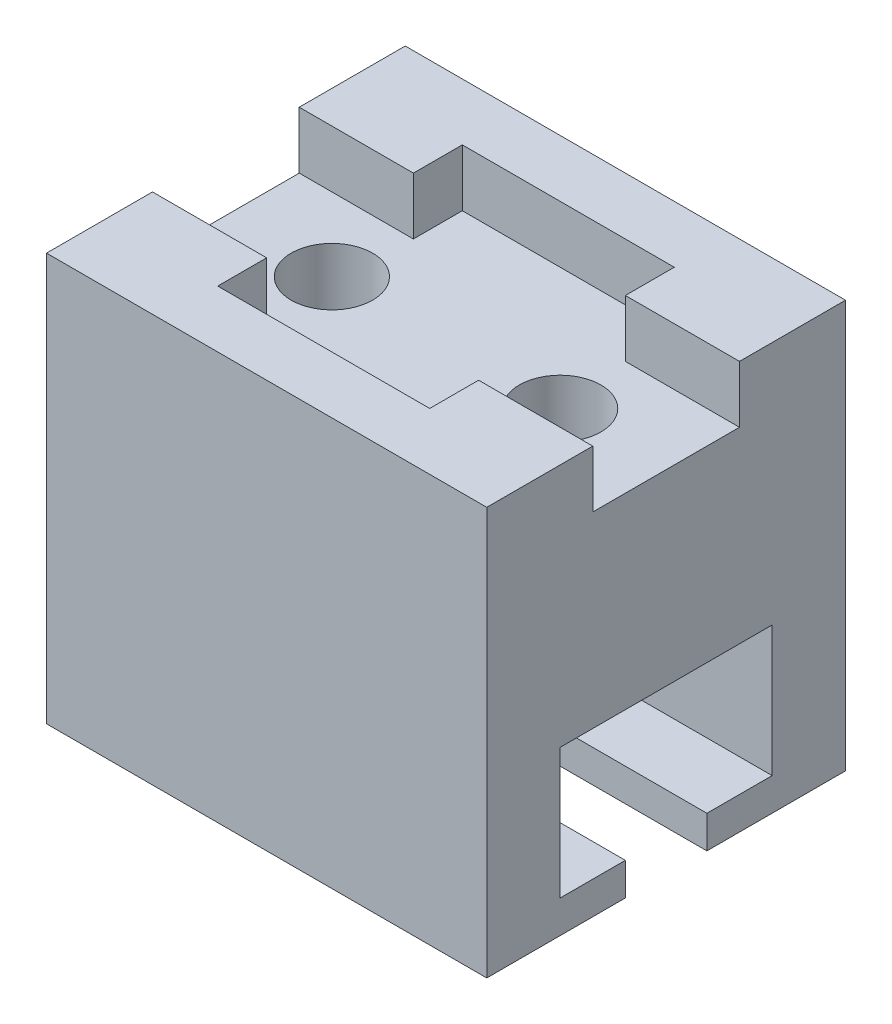
ISO-10303-21;
HEADER;
FILE_DESCRIPTION(('STEP AP214'),'2;1');
FILE_NAME('part.step','',(''),(''),'','','');
FILE_SCHEMA(('AUTOMOTIVE_DESIGN { 1 0 10303 214 1 1 1 1 }'));
ENDSEC;
DATA;
#1=APPLICATION_CONTEXT('core data for automotive mechanical design processes');
#2=APPLICATION_PROTOCOL_DEFINITION('international standard','automotive_design',2000,#1);
#3=PRODUCT_CONTEXT('',#1,'mechanical');
#4=PRODUCT('Part','Part','',(#3));
#5=PRODUCT_RELATED_PRODUCT_CATEGORY('part','',(#4));
#6=PRODUCT_DEFINITION_FORMATION('','',#4);
#7=PRODUCT_DEFINITION_CONTEXT('part definition',#1,'design');
#8=PRODUCT_DEFINITION('design','',#6,#7);
#9=PRODUCT_DEFINITION_SHAPE('','',#8);
#10=(LENGTH_UNIT() NAMED_UNIT(*) SI_UNIT(.MILLI.,.METRE.));
#11=(NAMED_UNIT(*) PLANE_ANGLE_UNIT() SI_UNIT($,.RADIAN.));
#12=(NAMED_UNIT(*) SI_UNIT($,.STERADIAN.) SOLID_ANGLE_UNIT());
#13=UNCERTAINTY_MEASURE_WITH_UNIT(LENGTH_MEASURE(1.E-05),#10,'distance_accuracy_value','');
#14=(GEOMETRIC_REPRESENTATION_CONTEXT(3) GLOBAL_UNCERTAINTY_ASSIGNED_CONTEXT((#13)) GLOBAL_UNIT_ASSIGNED_CONTEXT((#10,
#11,#12)) REPRESENTATION_CONTEXT('',''));
#15=CARTESIAN_POINT('',(0.,0.,0.));
#16=DIRECTION('',(0.,0.,1.));
#17=DIRECTION('',(1.,0.,0.));
#18=AXIS2_PLACEMENT_3D('',#15,#16,#17);
#19=CARTESIAN_POINT('',(-27.,-25.,-44.));
#20=DIRECTION('',(0.,-1.,0.));
#21=DIRECTION('',(0.,0.,-1.));
#22=AXIS2_PLACEMENT_3D('',#19,#20,#21);
#23=PLANE('',#22);
#24=DIRECTION('',(-1.,0.,0.));
#25=VECTOR('',#24,1.);
#26=CARTESIAN_POINT('',(27.,-25.,-27.));
#27=LINE('',#26,#25);
#28=CARTESIAN_POINT('',(27.,-25.,-27.));
#29=VERTEX_POINT('',#28);
#30=CARTESIAN_POINT('',(-27.,-25.,-27.));
#31=VERTEX_POINT('',#30);
#32=EDGE_CURVE('E325',#29,#31,#27,.T.);
#33=ORIENTED_EDGE('',*,*,#32,.T.);
#34=DIRECTION('',(0.,0.,1.));
#35=VECTOR('',#34,1.);
#36=CARTESIAN_POINT('',(-27.,-25.,-44.));
#37=LINE('',#36,#35);
#38=CARTESIAN_POINT('',(-27.,-25.,-44.));
#39=VERTEX_POINT('',#38);
#40=EDGE_CURVE('E223',#39,#31,#37,.T.);
#41=ORIENTED_EDGE('',*,*,#40,.F.);
#42=DIRECTION('',(1.,0.,0.));
#43=VECTOR('',#42,1.);
#44=CARTESIAN_POINT('',(-27.,-25.,-44.));
#45=LINE('',#44,#43);
#46=CARTESIAN_POINT('',(27.,-25.,-44.));
#47=VERTEX_POINT('',#46);
#48=EDGE_CURVE('E248',#39,#47,#45,.T.);
#49=ORIENTED_EDGE('',*,*,#48,.T.);
#50=DIRECTION('',(0.,0.,1.));
#51=VECTOR('',#50,1.);
#52=CARTESIAN_POINT('',(27.,-25.,-44.));
#53=LINE('',#52,#51);
#54=EDGE_CURVE('E11',#47,#29,#53,.T.);
#55=ORIENTED_EDGE('',*,*,#54,.T.);
#56=EDGE_LOOP('',(#33,#41,#49,#55));
#57=FACE_BOUND('',#56,.T.);
#58=ADVANCED_FACE('F41',(#57),#23,.T.);
#59=CARTESIAN_POINT('',(-27.,25.,-44.));
#60=DIRECTION('',(0.,1.,0.));
#61=DIRECTION('',(0.,0.,1.));
#62=AXIS2_PLACEMENT_3D('',#59,#60,#61);
#63=PLANE('',#62);
#64=DIRECTION('',(1.,0.,0.));
#65=VECTOR('',#64,1.);
#66=CARTESIAN_POINT('',(13.,25.,-13.));
#67=LINE('',#66,#65);
#68=CARTESIAN_POINT('',(13.,25.,-13.));
#69=VERTEX_POINT('',#68);
#70=CARTESIAN_POINT('',(27.,25.,-13.));
#71=VERTEX_POINT('',#70);
#72=EDGE_CURVE('E300',#69,#71,#67,.T.);
#73=ORIENTED_EDGE('',*,*,#72,.F.);
#74=DIRECTION('',(0.,0.,-1.));
#75=VECTOR('',#74,1.);
#76=CARTESIAN_POINT('',(13.,25.,-7.));
#77=LINE('',#76,#75);
#78=CARTESIAN_POINT('',(13.,25.,-7.));
#79=VERTEX_POINT('',#78);
#80=EDGE_CURVE('E303',#79,#69,#77,.T.);
#81=ORIENTED_EDGE('',*,*,#80,.F.);
#82=DIRECTION('',(1.,0.,0.));
#83=VECTOR('',#82,1.);
#84=CARTESIAN_POINT('',(-13.,25.,-7.));
#85=LINE('',#84,#83);
#86=CARTESIAN_POINT('',(-13.,25.,-7.));
#87=VERTEX_POINT('',#86);
#88=EDGE_CURVE('E305',#87,#79,#85,.T.);
#89=ORIENTED_EDGE('',*,*,#88,.F.);
#90=DIRECTION('',(0.,0.,1.));
#91=VECTOR('',#90,1.);
#92=CARTESIAN_POINT('',(-13.,25.,-7.));
#93=LINE('',#92,#91);
#94=CARTESIAN_POINT('',(-13.,25.,-13.));
#95=VERTEX_POINT('',#94);
#96=EDGE_CURVE('E307',#95,#87,#93,.T.);
#97=ORIENTED_EDGE('',*,*,#96,.F.);
#98=DIRECTION('',(1.,0.,0.));
#99=VECTOR('',#98,1.);
#100=CARTESIAN_POINT('',(-27.,25.,-13.));
#101=LINE('',#100,#99);
#102=CARTESIAN_POINT('',(-27.,25.,-13.));
#103=VERTEX_POINT('',#102);
#104=EDGE_CURVE('E309',#103,#95,#101,.T.);
#105=ORIENTED_EDGE('',*,*,#104,.F.);
#106=DIRECTION('',(0.,0.,1.));
#107=VECTOR('',#106,1.);
#108=CARTESIAN_POINT('',(-27.,25.,-44.));
#109=LINE('',#108,#107);
#110=CARTESIAN_POINT('',(-27.,25.,0.));
#111=VERTEX_POINT('',#110);
#112=EDGE_CURVE('E232',#103,#111,#109,.T.);
#113=ORIENTED_EDGE('',*,*,#112,.T.);
#114=DIRECTION('',(-1.,0.,0.));
#115=VECTOR('',#114,1.);
#116=CARTESIAN_POINT('',(-27.,25.,0.));
#117=LINE('',#116,#115);
#118=CARTESIAN_POINT('',(27.,25.,0.));
#119=VERTEX_POINT('',#118);
#120=EDGE_CURVE('E257',#119,#111,#117,.T.);
#121=ORIENTED_EDGE('',*,*,#120,.F.);
#122=DIRECTION('',(0.,0.,1.));
#123=VECTOR('',#122,1.);
#124=CARTESIAN_POINT('',(27.,25.,-44.));
#125=LINE('',#124,#123);
#126=EDGE_CURVE('E242',#71,#119,#125,.T.);
#127=ORIENTED_EDGE('',*,*,#126,.F.);
#128=EDGE_LOOP('',(#73,#81,#89,#97,#105,#113,#121,#127));
#129=FACE_BOUND('',#128,.T.);
#130=ADVANCED_FACE('F448',(#129),#63,.T.);
#131=CARTESIAN_POINT('',(27.,-25.,-44.));
#132=DIRECTION('',(1.,0.,0.));
#133=DIRECTION('',(0.,0.,-1.));
#134=AXIS2_PLACEMENT_3D('',#131,#132,#133);
#135=PLANE('',#134);
#136=DIRECTION('',(0.,-1.,0.));
#137=VECTOR('',#136,1.);
#138=CARTESIAN_POINT('',(27.,-25.,-27.));
#139=LINE('',#138,#137);
#140=CARTESIAN_POINT('',(27.,-21.,-27.));
#141=VERTEX_POINT('',#140);
#142=EDGE_CURVE('E218',#141,#29,#139,.T.);
#143=ORIENTED_EDGE('',*,*,#142,.T.);
#144=ORIENTED_EDGE('',*,*,#54,.F.);
#145=DIRECTION('',(0.,1.,0.));
#146=VECTOR('',#145,1.);
#147=CARTESIAN_POINT('',(27.,-25.,-44.));
#148=LINE('',#147,#146);
#149=CARTESIAN_POINT('',(27.,25.,-44.));
#150=VERTEX_POINT('',#149);
#151=EDGE_CURVE('E266',#47,#150,#148,.T.);
#152=ORIENTED_EDGE('',*,*,#151,.T.);
#153=CARTESIAN_POINT('',(27.,25.,-31.));
#154=VERTEX_POINT('',#153);
#155=EDGE_CURVE('E44',#150,#154,#125,.T.);
#156=ORIENTED_EDGE('',*,*,#155,.T.);
#157=DIRECTION('',(0.,1.,0.));
#158=VECTOR('',#157,1.);
#159=CARTESIAN_POINT('',(27.,18.,-31.));
#160=LINE('',#159,#158);
#161=CARTESIAN_POINT('',(27.,18.,-31.));
#162=VERTEX_POINT('',#161);
#163=EDGE_CURVE('E295',#162,#154,#160,.T.);
#164=ORIENTED_EDGE('',*,*,#163,.F.);
#165=DIRECTION('',(0.,0.,-1.));
#166=VECTOR('',#165,1.);
#167=CARTESIAN_POINT('',(27.,18.,-31.));
#168=LINE('',#167,#166);
#169=CARTESIAN_POINT('',(27.,18.,-13.));
#170=VERTEX_POINT('',#169);
#171=EDGE_CURVE('E324',#170,#162,#168,.T.);
#172=ORIENTED_EDGE('',*,*,#171,.F.);
#173=DIRECTION('',(0.,1.,0.));
#174=VECTOR('',#173,1.);
#175=CARTESIAN_POINT('',(27.,18.,-13.));
#176=LINE('',#175,#174);
#177=EDGE_CURVE('E286',#170,#71,#176,.T.);
#178=ORIENTED_EDGE('',*,*,#177,.T.);
#179=ORIENTED_EDGE('',*,*,#126,.T.);
#180=DIRECTION('',(0.,1.,0.));
#181=VECTOR('',#180,1.);
#182=CARTESIAN_POINT('',(27.,-25.,0.));
#183=LINE('',#182,#181);
#184=CARTESIAN_POINT('',(27.,-25.,0.));
#185=VERTEX_POINT('',#184);
#186=EDGE_CURVE('E224',#185,#119,#183,.T.);
#187=ORIENTED_EDGE('',*,*,#186,.F.);
#188=CARTESIAN_POINT('',(27.,-25.,-17.));
#189=VERTEX_POINT('',#188);
#190=EDGE_CURVE('E49',#189,#185,#53,.T.);
#191=ORIENTED_EDGE('',*,*,#190,.F.);
#192=DIRECTION('',(0.,1.,0.));
#193=VECTOR('',#192,1.);
#194=CARTESIAN_POINT('',(27.,-21.,-17.));
#195=LINE('',#194,#193);
#196=CARTESIAN_POINT('',(27.,-21.,-17.));
#197=VERTEX_POINT('',#196);
#198=EDGE_CURVE('E201',#189,#197,#195,.T.);
#199=ORIENTED_EDGE('',*,*,#198,.T.);
#200=DIRECTION('',(0.,0.,1.));
#201=VECTOR('',#200,1.);
#202=CARTESIAN_POINT('',(27.,-21.,-9.));
#203=LINE('',#202,#201);
#204=CARTESIAN_POINT('',(27.,-21.,-9.));
#205=VERTEX_POINT('',#204);
#206=EDGE_CURVE('E209',#197,#205,#203,.T.);
#207=ORIENTED_EDGE('',*,*,#206,.T.);
#208=DIRECTION('',(0.,1.,0.));
#209=VECTOR('',#208,1.);
#210=CARTESIAN_POINT('',(27.,-5.,-9.));
#211=LINE('',#210,#209);
#212=CARTESIAN_POINT('',(27.,-5.,-9.));
#213=VERTEX_POINT('',#212);
#214=EDGE_CURVE('E397',#205,#213,#211,.T.);
#215=ORIENTED_EDGE('',*,*,#214,.T.);
#216=DIRECTION('',(0.,0.,-1.));
#217=VECTOR('',#216,1.);
#218=CARTESIAN_POINT('',(27.,-5.,-35.));
#219=LINE('',#218,#217);
#220=CARTESIAN_POINT('',(27.,-5.,-35.));
#221=VERTEX_POINT('',#220);
#222=EDGE_CURVE('E391',#213,#221,#219,.T.);
#223=ORIENTED_EDGE('',*,*,#222,.T.);
#224=DIRECTION('',(0.,-1.,0.));
#225=VECTOR('',#224,1.);
#226=CARTESIAN_POINT('',(27.,-21.,-35.));
#227=LINE('',#226,#225);
#228=CARTESIAN_POINT('',(27.,-21.,-35.));
#229=VERTEX_POINT('',#228);
#230=EDGE_CURVE('E394',#221,#229,#227,.T.);
#231=ORIENTED_EDGE('',*,*,#230,.T.);
#232=DIRECTION('',(0.,0.,1.));
#233=VECTOR('',#232,1.);
#234=CARTESIAN_POINT('',(27.,-21.,-27.));
#235=LINE('',#234,#233);
#236=EDGE_CURVE('E386',#229,#141,#235,.T.);
#237=ORIENTED_EDGE('',*,*,#236,.T.);
#238=EDGE_LOOP('',(#143,#144,#152,#156,#164,#172,#178,#179,#187,#191,#199,#207,#215,#223,#231,#237));
#239=FACE_BOUND('',#238,.T.);
#240=ADVANCED_FACE('F43',(#239),#135,.T.);
#241=DIRECTION('',(-1.,0.,0.));
#242=VECTOR('',#241,1.);
#243=CARTESIAN_POINT('',(27.,-25.,-17.));
#244=LINE('',#243,#242);
#245=CARTESIAN_POINT('',(-27.,-25.,-17.));
#246=VERTEX_POINT('',#245);
#247=EDGE_CURVE('E59',#189,#246,#244,.T.);
#248=ORIENTED_EDGE('',*,*,#247,.F.);
#249=ORIENTED_EDGE('',*,*,#190,.T.);
#250=DIRECTION('',(1.,0.,0.));
#251=VECTOR('',#250,1.);
#252=CARTESIAN_POINT('',(-27.,-25.,0.));
#253=LINE('',#252,#251);
#254=CARTESIAN_POINT('',(-27.,-25.,0.));
#255=VERTEX_POINT('',#254);
#256=EDGE_CURVE('E230',#255,#185,#253,.T.);
#257=ORIENTED_EDGE('',*,*,#256,.F.);
#258=EDGE_CURVE('E217',#246,#255,#37,.T.);
#259=ORIENTED_EDGE('',*,*,#258,.F.);
#260=EDGE_LOOP('',(#248,#249,#257,#259));
#261=FACE_BOUND('',#260,.T.);
#262=ADVANCED_FACE('F214',(#261),#23,.T.);
#263=CARTESIAN_POINT('',(-27.,-25.,-44.));
#264=DIRECTION('',(-1.,0.,0.));
#265=DIRECTION('',(0.,0.,1.));
#266=AXIS2_PLACEMENT_3D('',#263,#264,#265);
#267=PLANE('',#266);
#268=DIRECTION('',(0.,-1.,0.));
#269=VECTOR('',#268,1.);
#270=CARTESIAN_POINT('',(-27.,-25.,-27.));
#271=LINE('',#270,#269);
#272=CARTESIAN_POINT('',(-27.,-21.,-27.));
#273=VERTEX_POINT('',#272);
#274=EDGE_CURVE('E211',#273,#31,#271,.T.);
#275=ORIENTED_EDGE('',*,*,#274,.F.);
#276=DIRECTION('',(0.,0.,1.));
#277=VECTOR('',#276,1.);
#278=CARTESIAN_POINT('',(-27.,-21.,-27.));
#279=LINE('',#278,#277);
#280=CARTESIAN_POINT('',(-27.,-21.,-35.));
#281=VERTEX_POINT('',#280);
#282=EDGE_CURVE('E367',#281,#273,#279,.T.);
#283=ORIENTED_EDGE('',*,*,#282,.F.);
#284=DIRECTION('',(0.,-1.,0.));
#285=VECTOR('',#284,1.);
#286=CARTESIAN_POINT('',(-27.,-21.,-35.));
#287=LINE('',#286,#285);
#288=CARTESIAN_POINT('',(-27.,-5.,-35.));
#289=VERTEX_POINT('',#288);
#290=EDGE_CURVE('E373',#289,#281,#287,.T.);
#291=ORIENTED_EDGE('',*,*,#290,.F.);
#292=DIRECTION('',(0.,0.,-1.));
#293=VECTOR('',#292,1.);
#294=CARTESIAN_POINT('',(-27.,-5.,-35.));
#295=LINE('',#294,#293);
#296=CARTESIAN_POINT('',(-27.,-5.,-9.));
#297=VERTEX_POINT('',#296);
#298=EDGE_CURVE('E376',#297,#289,#295,.T.);
#299=ORIENTED_EDGE('',*,*,#298,.F.);
#300=DIRECTION('',(0.,1.,0.));
#301=VECTOR('',#300,1.);
#302=CARTESIAN_POINT('',(-27.,-5.,-9.));
#303=LINE('',#302,#301);
#304=CARTESIAN_POINT('',(-27.,-21.,-9.));
#305=VERTEX_POINT('',#304);
#306=EDGE_CURVE('E377',#305,#297,#303,.T.);
#307=ORIENTED_EDGE('',*,*,#306,.F.);
#308=DIRECTION('',(0.,0.,1.));
#309=VECTOR('',#308,1.);
#310=CARTESIAN_POINT('',(-27.,-21.,-9.));
#311=LINE('',#310,#309);
#312=CARTESIAN_POINT('',(-27.,-21.,-17.));
#313=VERTEX_POINT('',#312);
#314=EDGE_CURVE('E385',#313,#305,#311,.T.);
#315=ORIENTED_EDGE('',*,*,#314,.F.);
#316=DIRECTION('',(0.,1.,0.));
#317=VECTOR('',#316,1.);
#318=CARTESIAN_POINT('',(-27.,-21.,-17.));
#319=LINE('',#318,#317);
#320=EDGE_CURVE('E384',#246,#313,#319,.T.);
#321=ORIENTED_EDGE('',*,*,#320,.F.);
#322=ORIENTED_EDGE('',*,*,#258,.T.);
#323=DIRECTION('',(0.,-1.,0.));
#324=VECTOR('',#323,1.);
#325=CARTESIAN_POINT('',(-27.,-25.,0.));
#326=LINE('',#325,#324);
#327=EDGE_CURVE('E263',#111,#255,#326,.T.);
#328=ORIENTED_EDGE('',*,*,#327,.F.);
#329=ORIENTED_EDGE('',*,*,#112,.F.);
#330=DIRECTION('',(0.,1.,0.));
#331=VECTOR('',#330,1.);
#332=CARTESIAN_POINT('',(-27.,18.,-13.));
#333=LINE('',#332,#331);
#334=CARTESIAN_POINT('',(-27.,18.,-13.));
#335=VERTEX_POINT('',#334);
#336=EDGE_CURVE('E278',#335,#103,#333,.T.);
#337=ORIENTED_EDGE('',*,*,#336,.F.);
#338=DIRECTION('',(0.,0.,1.));
#339=VECTOR('',#338,1.);
#340=CARTESIAN_POINT('',(-27.,18.,-31.));
#341=LINE('',#340,#339);
#342=CARTESIAN_POINT('',(-27.,18.,-31.));
#343=VERTEX_POINT('',#342);
#344=EDGE_CURVE('E344',#343,#335,#341,.T.);
#345=ORIENTED_EDGE('',*,*,#344,.F.);
#346=DIRECTION('',(0.,1.,0.));
#347=VECTOR('',#346,1.);
#348=CARTESIAN_POINT('',(-27.,18.,-31.));
#349=LINE('',#348,#347);
#350=CARTESIAN_POINT('',(-27.,25.,-31.));
#351=VERTEX_POINT('',#350);
#352=EDGE_CURVE('E280',#343,#351,#349,.T.);
#353=ORIENTED_EDGE('',*,*,#352,.T.);
#354=CARTESIAN_POINT('',(-27.,25.,-44.));
#355=VERTEX_POINT('',#354);
#356=EDGE_CURVE('E233',#355,#351,#109,.T.);
#357=ORIENTED_EDGE('',*,*,#356,.F.);
#358=DIRECTION('',(0.,-1.,0.));
#359=VECTOR('',#358,1.);
#360=CARTESIAN_POINT('',(-27.,-25.,-44.));
#361=LINE('',#360,#359);
#362=EDGE_CURVE('E246',#355,#39,#361,.T.);
#363=ORIENTED_EDGE('',*,*,#362,.T.);
#364=ORIENTED_EDGE('',*,*,#40,.T.);
#365=EDGE_LOOP('',(#275,#283,#291,#299,#307,#315,#321,#322,#328,#329,#337,#345,#353,#357,#363,#364));
#366=FACE_BOUND('',#365,.T.);
#367=ADVANCED_FACE('F442',(#366),#267,.T.);
#368=DIRECTION('',(-1.,0.,0.));
#369=VECTOR('',#368,1.);
#370=CARTESIAN_POINT('',(13.,25.,-31.));
#371=LINE('',#370,#369);
#372=CARTESIAN_POINT('',(13.,25.,-31.));
#373=VERTEX_POINT('',#372);
#374=EDGE_CURVE('E293',#154,#373,#371,.T.);
#375=ORIENTED_EDGE('',*,*,#374,.F.);
#376=ORIENTED_EDGE('',*,*,#155,.F.);
#377=DIRECTION('',(-1.,0.,0.));
#378=VECTOR('',#377,1.);
#379=CARTESIAN_POINT('',(-27.,25.,-44.));
#380=LINE('',#379,#378);
#381=EDGE_CURVE('E254',#150,#355,#380,.T.);
#382=ORIENTED_EDGE('',*,*,#381,.T.);
#383=ORIENTED_EDGE('',*,*,#356,.T.);
#384=DIRECTION('',(-1.,0.,0.));
#385=VECTOR('',#384,1.);
#386=CARTESIAN_POINT('',(-27.,25.,-31.));
#387=LINE('',#386,#385);
#388=CARTESIAN_POINT('',(-13.,25.,-31.));
#389=VERTEX_POINT('',#388);
#390=EDGE_CURVE('E311',#389,#351,#387,.T.);
#391=ORIENTED_EDGE('',*,*,#390,.F.);
#392=DIRECTION('',(0.,0.,1.));
#393=VECTOR('',#392,1.);
#394=CARTESIAN_POINT('',(-13.,25.,-37.));
#395=LINE('',#394,#393);
#396=CARTESIAN_POINT('',(-13.,25.,-37.));
#397=VERTEX_POINT('',#396);
#398=EDGE_CURVE('E312',#397,#389,#395,.T.);
#399=ORIENTED_EDGE('',*,*,#398,.F.);
#400=DIRECTION('',(-1.,0.,0.));
#401=VECTOR('',#400,1.);
#402=CARTESIAN_POINT('',(-13.,25.,-37.));
#403=LINE('',#402,#401);
#404=CARTESIAN_POINT('',(13.,25.,-37.));
#405=VERTEX_POINT('',#404);
#406=EDGE_CURVE('E318',#405,#397,#403,.T.);
#407=ORIENTED_EDGE('',*,*,#406,.F.);
#408=DIRECTION('',(0.,0.,-1.));
#409=VECTOR('',#408,1.);
#410=CARTESIAN_POINT('',(13.,25.,-37.));
#411=LINE('',#410,#409);
#412=EDGE_CURVE('E68',#373,#405,#411,.T.);
#413=ORIENTED_EDGE('',*,*,#412,.F.);
#414=EDGE_LOOP('',(#375,#376,#382,#383,#391,#399,#407,#413));
#415=FACE_BOUND('',#414,.T.);
#416=ADVANCED_FACE('F461',(#415),#63,.T.);
#417=CARTESIAN_POINT('',(0.,0.,-44.));
#418=DIRECTION('',(0.,0.,-1.));
#419=DIRECTION('',(-1.,0.,0.));
#420=AXIS2_PLACEMENT_3D('',#417,#418,#419);
#421=PLANE('',#420);
#422=ORIENTED_EDGE('',*,*,#151,.F.);
#423=ORIENTED_EDGE('',*,*,#48,.F.);
#424=ORIENTED_EDGE('',*,*,#362,.F.);
#425=ORIENTED_EDGE('',*,*,#381,.F.);
#426=EDGE_LOOP('',(#422,#423,#424,#425));
#427=FACE_BOUND('',#426,.T.);
#428=ADVANCED_FACE('F640',(#427),#421,.T.);
#429=CARTESIAN_POINT('',(0.,0.,0.));
#430=DIRECTION('',(0.,0.,-1.));
#431=DIRECTION('',(-1.,0.,0.));
#432=AXIS2_PLACEMENT_3D('',#429,#430,#431);
#433=PLANE('',#432);
#434=ORIENTED_EDGE('',*,*,#186,.T.);
#435=ORIENTED_EDGE('',*,*,#120,.T.);
#436=ORIENTED_EDGE('',*,*,#327,.T.);
#437=ORIENTED_EDGE('',*,*,#256,.T.);
#438=EDGE_LOOP('',(#434,#435,#436,#437));
#439=FACE_BOUND('',#438,.T.);
#440=ADVANCED_FACE('F636',(#439),#433,.F.);
#441=CARTESIAN_POINT('',(13.,18.,-37.));
#442=DIRECTION('',(1.,0.,0.));
#443=DIRECTION('',(0.,0.,-1.));
#444=AXIS2_PLACEMENT_3D('',#441,#442,#443);
#445=PLANE('',#444);
#446=ORIENTED_EDGE('',*,*,#412,.T.);
#447=DIRECTION('',(0.,1.,0.));
#448=VECTOR('',#447,1.);
#449=CARTESIAN_POINT('',(13.,18.,-37.));
#450=LINE('',#449,#448);
#451=CARTESIAN_POINT('',(13.,18.,-37.));
#452=VERTEX_POINT('',#451);
#453=EDGE_CURVE('E269',#452,#405,#450,.T.);
#454=ORIENTED_EDGE('',*,*,#453,.F.);
#455=DIRECTION('',(0.,0.,-1.));
#456=VECTOR('',#455,1.);
#457=CARTESIAN_POINT('',(13.,18.,-37.));
#458=LINE('',#457,#456);
#459=CARTESIAN_POINT('',(13.,18.,-31.));
#460=VERTEX_POINT('',#459);
#461=EDGE_CURVE('E297',#460,#452,#458,.T.);
#462=ORIENTED_EDGE('',*,*,#461,.F.);
#463=DIRECTION('',(0.,1.,0.));
#464=VECTOR('',#463,1.);
#465=CARTESIAN_POINT('',(13.,18.,-31.));
#466=LINE('',#465,#464);
#467=EDGE_CURVE('E261',#460,#373,#466,.T.);
#468=ORIENTED_EDGE('',*,*,#467,.T.);
#469=EDGE_LOOP('',(#446,#454,#462,#468));
#470=FACE_BOUND('',#469,.T.);
#471=ADVANCED_FACE('F428',(#470),#445,.F.);
#472=CARTESIAN_POINT('',(13.,18.,-31.));
#473=DIRECTION('',(0.,0.,-1.));
#474=DIRECTION('',(-1.,0.,0.));
#475=AXIS2_PLACEMENT_3D('',#472,#473,#474);
#476=PLANE('',#475);
#477=ORIENTED_EDGE('',*,*,#374,.T.);
#478=ORIENTED_EDGE('',*,*,#467,.F.);
#479=DIRECTION('',(-1.,0.,0.));
#480=VECTOR('',#479,1.);
#481=CARTESIAN_POINT('',(13.,18.,-31.));
#482=LINE('',#481,#480);
#483=EDGE_CURVE('E272',#162,#460,#482,.T.);
#484=ORIENTED_EDGE('',*,*,#483,.F.);
#485=ORIENTED_EDGE('',*,*,#163,.T.);
#486=EDGE_LOOP('',(#477,#478,#484,#485));
#487=FACE_BOUND('',#486,.T.);
#488=ADVANCED_FACE('F465',(#487),#476,.F.);
#489=CARTESIAN_POINT('',(13.,18.,-13.));
#490=DIRECTION('',(0.,0.,1.));
#491=DIRECTION('',(1.,0.,0.));
#492=AXIS2_PLACEMENT_3D('',#489,#490,#491);
#493=PLANE('',#492);
#494=ORIENTED_EDGE('',*,*,#72,.T.);
#495=ORIENTED_EDGE('',*,*,#177,.F.);
#496=DIRECTION('',(1.,0.,0.));
#497=VECTOR('',#496,1.);
#498=CARTESIAN_POINT('',(13.,18.,-13.));
#499=LINE('',#498,#497);
#500=CARTESIAN_POINT('',(13.,18.,-13.));
#501=VERTEX_POINT('',#500);
#502=EDGE_CURVE('E330',#501,#170,#499,.T.);
#503=ORIENTED_EDGE('',*,*,#502,.F.);
#504=DIRECTION('',(0.,1.,0.));
#505=VECTOR('',#504,1.);
#506=CARTESIAN_POINT('',(13.,18.,-13.));
#507=LINE('',#506,#505);
#508=EDGE_CURVE('E287',#501,#69,#507,.T.);
#509=ORIENTED_EDGE('',*,*,#508,.T.);
#510=EDGE_LOOP('',(#494,#495,#503,#509));
#511=FACE_BOUND('',#510,.T.);
#512=ADVANCED_FACE('F458',(#511),#493,.F.);
#513=CARTESIAN_POINT('',(13.,18.,-7.));
#514=DIRECTION('',(1.,0.,0.));
#515=DIRECTION('',(0.,0.,-1.));
#516=AXIS2_PLACEMENT_3D('',#513,#514,#515);
#517=PLANE('',#516);
#518=ORIENTED_EDGE('',*,*,#80,.T.);
#519=ORIENTED_EDGE('',*,*,#508,.F.);
#520=DIRECTION('',(0.,0.,-1.));
#521=VECTOR('',#520,1.);
#522=CARTESIAN_POINT('',(13.,18.,-7.));
#523=LINE('',#522,#521);
#524=CARTESIAN_POINT('',(13.,18.,-7.));
#525=VERTEX_POINT('',#524);
#526=EDGE_CURVE('E329',#525,#501,#523,.T.);
#527=ORIENTED_EDGE('',*,*,#526,.F.);
#528=DIRECTION('',(0.,1.,0.));
#529=VECTOR('',#528,1.);
#530=CARTESIAN_POINT('',(13.,18.,-7.));
#531=LINE('',#530,#529);
#532=EDGE_CURVE('E288',#525,#79,#531,.T.);
#533=ORIENTED_EDGE('',*,*,#532,.T.);
#534=EDGE_LOOP('',(#518,#519,#527,#533));
#535=FACE_BOUND('',#534,.T.);
#536=ADVANCED_FACE('F460',(#535),#517,.F.);
#537=CARTESIAN_POINT('',(-13.,18.,-7.));
#538=DIRECTION('',(0.,0.,1.));
#539=DIRECTION('',(1.,0.,0.));
#540=AXIS2_PLACEMENT_3D('',#537,#538,#539);
#541=PLANE('',#540);
#542=ORIENTED_EDGE('',*,*,#88,.T.);
#543=ORIENTED_EDGE('',*,*,#532,.F.);
#544=DIRECTION('',(1.,0.,0.));
#545=VECTOR('',#544,1.);
#546=CARTESIAN_POINT('',(-13.,18.,-7.));
#547=LINE('',#546,#545);
#548=CARTESIAN_POINT('',(-13.,18.,-7.));
#549=VERTEX_POINT('',#548);
#550=EDGE_CURVE('E334',#549,#525,#547,.T.);
#551=ORIENTED_EDGE('',*,*,#550,.F.);
#552=DIRECTION('',(0.,1.,0.));
#553=VECTOR('',#552,1.);
#554=CARTESIAN_POINT('',(-13.,18.,-7.));
#555=LINE('',#554,#553);
#556=EDGE_CURVE('E285',#549,#87,#555,.T.);
#557=ORIENTED_EDGE('',*,*,#556,.T.);
#558=EDGE_LOOP('',(#542,#543,#551,#557));
#559=FACE_BOUND('',#558,.T.);
#560=ADVANCED_FACE('F451',(#559),#541,.F.);
#561=CARTESIAN_POINT('',(-13.,18.,-7.));
#562=DIRECTION('',(-1.,0.,0.));
#563=DIRECTION('',(0.,0.,1.));
#564=AXIS2_PLACEMENT_3D('',#561,#562,#563);
#565=PLANE('',#564);
#566=ORIENTED_EDGE('',*,*,#96,.T.);
#567=ORIENTED_EDGE('',*,*,#556,.F.);
#568=DIRECTION('',(0.,0.,1.));
#569=VECTOR('',#568,1.);
#570=CARTESIAN_POINT('',(-13.,18.,-7.));
#571=LINE('',#570,#569);
#572=CARTESIAN_POINT('',(-13.,18.,-13.));
#573=VERTEX_POINT('',#572);
#574=EDGE_CURVE('E338',#573,#549,#571,.T.);
#575=ORIENTED_EDGE('',*,*,#574,.F.);
#576=DIRECTION('',(0.,1.,0.));
#577=VECTOR('',#576,1.);
#578=CARTESIAN_POINT('',(-13.,18.,-13.));
#579=LINE('',#578,#577);
#580=EDGE_CURVE('E284',#573,#95,#579,.T.);
#581=ORIENTED_EDGE('',*,*,#580,.T.);
#582=EDGE_LOOP('',(#566,#567,#575,#581));
#583=FACE_BOUND('',#582,.T.);
#584=ADVANCED_FACE('F446',(#583),#565,.F.);
#585=CARTESIAN_POINT('',(-27.,18.,-13.));
#586=DIRECTION('',(0.,0.,1.));
#587=DIRECTION('',(1.,0.,0.));
#588=AXIS2_PLACEMENT_3D('',#585,#586,#587);
#589=PLANE('',#588);
#590=ORIENTED_EDGE('',*,*,#104,.T.);
#591=ORIENTED_EDGE('',*,*,#580,.F.);
#592=DIRECTION('',(1.,0.,0.));
#593=VECTOR('',#592,1.);
#594=CARTESIAN_POINT('',(-27.,18.,-13.));
#595=LINE('',#594,#593);
#596=EDGE_CURVE('E340',#335,#573,#595,.T.);
#597=ORIENTED_EDGE('',*,*,#596,.F.);
#598=ORIENTED_EDGE('',*,*,#336,.T.);
#599=EDGE_LOOP('',(#590,#591,#597,#598));
#600=FACE_BOUND('',#599,.T.);
#601=ADVANCED_FACE('F444',(#600),#589,.F.);
#602=CARTESIAN_POINT('',(-27.,18.,-31.));
#603=DIRECTION('',(0.,0.,-1.));
#604=DIRECTION('',(-1.,0.,0.));
#605=AXIS2_PLACEMENT_3D('',#602,#603,#604);
#606=PLANE('',#605);
#607=ORIENTED_EDGE('',*,*,#390,.T.);
#608=ORIENTED_EDGE('',*,*,#352,.F.);
#609=DIRECTION('',(-1.,0.,0.));
#610=VECTOR('',#609,1.);
#611=CARTESIAN_POINT('',(-27.,18.,-31.));
#612=LINE('',#611,#610);
#613=CARTESIAN_POINT('',(-13.,18.,-31.));
#614=VERTEX_POINT('',#613);
#615=EDGE_CURVE('E341',#614,#343,#612,.T.);
#616=ORIENTED_EDGE('',*,*,#615,.F.);
#617=DIRECTION('',(0.,1.,0.));
#618=VECTOR('',#617,1.);
#619=CARTESIAN_POINT('',(-13.,18.,-31.));
#620=LINE('',#619,#618);
#621=EDGE_CURVE('E274',#614,#389,#620,.T.);
#622=ORIENTED_EDGE('',*,*,#621,.T.);
#623=EDGE_LOOP('',(#607,#608,#616,#622));
#624=FACE_BOUND('',#623,.T.);
#625=ADVANCED_FACE('F469',(#624),#606,.F.);
#626=CARTESIAN_POINT('',(-13.,18.,-37.));
#627=DIRECTION('',(-1.,0.,0.));
#628=DIRECTION('',(0.,0.,1.));
#629=AXIS2_PLACEMENT_3D('',#626,#627,#628);
#630=PLANE('',#629);
#631=ORIENTED_EDGE('',*,*,#398,.T.);
#632=ORIENTED_EDGE('',*,*,#621,.F.);
#633=DIRECTION('',(0.,0.,1.));
#634=VECTOR('',#633,1.);
#635=CARTESIAN_POINT('',(-13.,18.,-37.));
#636=LINE('',#635,#634);
#637=CARTESIAN_POINT('',(-13.,18.,-37.));
#638=VERTEX_POINT('',#637);
#639=EDGE_CURVE('E346',#638,#614,#636,.T.);
#640=ORIENTED_EDGE('',*,*,#639,.F.);
#641=DIRECTION('',(0.,1.,0.));
#642=VECTOR('',#641,1.);
#643=CARTESIAN_POINT('',(-13.,18.,-37.));
#644=LINE('',#643,#642);
#645=EDGE_CURVE('E275',#638,#397,#644,.T.);
#646=ORIENTED_EDGE('',*,*,#645,.T.);
#647=EDGE_LOOP('',(#631,#632,#640,#646));
#648=FACE_BOUND('',#647,.T.);
#649=ADVANCED_FACE('F432',(#648),#630,.F.);
#650=CARTESIAN_POINT('',(-13.,18.,-37.));
#651=DIRECTION('',(0.,0.,-1.));
#652=DIRECTION('',(-1.,0.,0.));
#653=AXIS2_PLACEMENT_3D('',#650,#651,#652);
#654=PLANE('',#653);
#655=ORIENTED_EDGE('',*,*,#406,.T.);
#656=ORIENTED_EDGE('',*,*,#645,.F.);
#657=DIRECTION('',(-1.,0.,0.));
#658=VECTOR('',#657,1.);
#659=CARTESIAN_POINT('',(-13.,18.,-37.));
#660=LINE('',#659,#658);
#661=EDGE_CURVE('E353',#452,#638,#660,.T.);
#662=ORIENTED_EDGE('',*,*,#661,.F.);
#663=ORIENTED_EDGE('',*,*,#453,.T.);
#664=EDGE_LOOP('',(#655,#656,#662,#663));
#665=FACE_BOUND('',#664,.T.);
#666=ADVANCED_FACE('F423',(#665),#654,.F.);
#667=CARTESIAN_POINT('',(0.,18.,0.));
#668=DIRECTION('',(0.,1.,0.));
#669=DIRECTION('',(0.,0.,1.));
#670=AXIS2_PLACEMENT_3D('',#667,#668,#669);
#671=PLANE('',#670);
#672=CARTESIAN_POINT('',(-14.,18.,-22.));
#673=DIRECTION('',(0.,1.,0.));
#674=DIRECTION('',(0.,0.,1.));
#675=AXIS2_PLACEMENT_3D('',#672,#673,#674);
#676=CIRCLE('',#675,5.);
#677=CARTESIAN_POINT('',(-14.,18.,-17.));
#678=VERTEX_POINT('',#677);
#679=EDGE_CURVE('E409',#678,#678,#676,.T.);
#680=ORIENTED_EDGE('',*,*,#679,.F.);
#681=EDGE_LOOP('',(#680));
#682=FACE_BOUND('',#681,.T.);
#683=CARTESIAN_POINT('',(14.,18.,-22.));
#684=DIRECTION('',(0.,1.,0.));
#685=DIRECTION('',(0.,0.,1.));
#686=AXIS2_PLACEMENT_3D('',#683,#684,#685);
#687=CIRCLE('',#686,5.);
#688=CARTESIAN_POINT('',(14.,18.,-17.));
#689=VERTEX_POINT('',#688);
#690=EDGE_CURVE('E407',#689,#689,#687,.T.);
#691=ORIENTED_EDGE('',*,*,#690,.F.);
#692=EDGE_LOOP('',(#691));
#693=FACE_BOUND('',#692,.T.);
#694=ORIENTED_EDGE('',*,*,#461,.T.);
#695=ORIENTED_EDGE('',*,*,#661,.T.);
#696=ORIENTED_EDGE('',*,*,#639,.T.);
#697=ORIENTED_EDGE('',*,*,#615,.T.);
#698=ORIENTED_EDGE('',*,*,#344,.T.);
#699=ORIENTED_EDGE('',*,*,#596,.T.);
#700=ORIENTED_EDGE('',*,*,#574,.T.);
#701=ORIENTED_EDGE('',*,*,#550,.T.);
#702=ORIENTED_EDGE('',*,*,#526,.T.);
#703=ORIENTED_EDGE('',*,*,#502,.T.);
#704=ORIENTED_EDGE('',*,*,#171,.T.);
#705=ORIENTED_EDGE('',*,*,#483,.T.);
#706=EDGE_LOOP('',(#694,#695,#696,#697,#698,#699,#700,#701,#702,#703,#704,#705));
#707=FACE_BOUND('',#706,.T.);
#708=ADVANCED_FACE('F417',(#682,#693,#707),#671,.T.);
#709=CARTESIAN_POINT('',(27.,-25.,-27.));
#710=DIRECTION('',(0.,0.,-1.));
#711=DIRECTION('',(-1.,0.,0.));
#712=AXIS2_PLACEMENT_3D('',#709,#710,#711);
#713=PLANE('',#712);
#714=ORIENTED_EDGE('',*,*,#274,.T.);
#715=ORIENTED_EDGE('',*,*,#32,.F.);
#716=ORIENTED_EDGE('',*,*,#142,.F.);
#717=DIRECTION('',(-1.,0.,0.));
#718=VECTOR('',#717,1.);
#719=CARTESIAN_POINT('',(27.,-21.,-27.));
#720=LINE('',#719,#718);
#721=EDGE_CURVE('E364',#141,#273,#720,.T.);
#722=ORIENTED_EDGE('',*,*,#721,.T.);
#723=EDGE_LOOP('',(#714,#715,#716,#722));
#724=FACE_BOUND('',#723,.T.);
#725=ADVANCED_FACE('F419',(#724),#713,.F.);
#726=CARTESIAN_POINT('',(27.,-21.,-27.));
#727=DIRECTION('',(0.,-1.,0.));
#728=DIRECTION('',(0.,0.,-1.));
#729=AXIS2_PLACEMENT_3D('',#726,#727,#728);
#730=PLANE('',#729);
#731=ORIENTED_EDGE('',*,*,#282,.T.);
#732=ORIENTED_EDGE('',*,*,#721,.F.);
#733=ORIENTED_EDGE('',*,*,#236,.F.);
#734=DIRECTION('',(-1.,0.,0.));
#735=VECTOR('',#734,1.);
#736=CARTESIAN_POINT('',(27.,-21.,-35.));
#737=LINE('',#736,#735);
#738=EDGE_CURVE('E361',#229,#281,#737,.T.);
#739=ORIENTED_EDGE('',*,*,#738,.T.);
#740=EDGE_LOOP('',(#731,#732,#733,#739));
#741=FACE_BOUND('',#740,.T.);
#742=ADVANCED_FACE('F507',(#741),#730,.F.);
#743=CARTESIAN_POINT('',(27.,-21.,-35.));
#744=DIRECTION('',(0.,0.,-1.));
#745=DIRECTION('',(-1.,0.,0.));
#746=AXIS2_PLACEMENT_3D('',#743,#744,#745);
#747=PLANE('',#746);
#748=ORIENTED_EDGE('',*,*,#290,.T.);
#749=ORIENTED_EDGE('',*,*,#738,.F.);
#750=ORIENTED_EDGE('',*,*,#230,.F.);
#751=DIRECTION('',(-1.,0.,0.));
#752=VECTOR('',#751,1.);
#753=CARTESIAN_POINT('',(27.,-5.,-35.));
#754=LINE('',#753,#752);
#755=EDGE_CURVE('E363',#221,#289,#754,.T.);
#756=ORIENTED_EDGE('',*,*,#755,.T.);
#757=EDGE_LOOP('',(#748,#749,#750,#756));
#758=FACE_BOUND('',#757,.T.);
#759=ADVANCED_FACE('F505',(#758),#747,.F.);
#760=CARTESIAN_POINT('',(27.,-5.,-35.));
#761=DIRECTION('',(0.,1.,0.));
#762=DIRECTION('',(0.,0.,1.));
#763=AXIS2_PLACEMENT_3D('',#760,#761,#762);
#764=PLANE('',#763);
#765=CARTESIAN_POINT('',(-14.,-5.,-22.));
#766=DIRECTION('',(0.,1.,0.));
#767=DIRECTION('',(0.,0.,1.));
#768=AXIS2_PLACEMENT_3D('',#765,#766,#767);
#769=CIRCLE('',#768,5.);
#770=CARTESIAN_POINT('',(-14.,-5.,-17.));
#771=VERTEX_POINT('',#770);
#772=EDGE_CURVE('E390',#771,#771,#769,.T.);
#773=ORIENTED_EDGE('',*,*,#772,.T.);
#774=EDGE_LOOP('',(#773));
#775=FACE_BOUND('',#774,.T.);
#776=CARTESIAN_POINT('',(14.,-5.,-22.));
#777=DIRECTION('',(0.,1.,0.));
#778=DIRECTION('',(0.,0.,1.));
#779=AXIS2_PLACEMENT_3D('',#776,#777,#778);
#780=CIRCLE('',#779,5.);
#781=CARTESIAN_POINT('',(14.,-5.,-17.));
#782=VERTEX_POINT('',#781);
#783=EDGE_CURVE('E404',#782,#782,#780,.T.);
#784=ORIENTED_EDGE('',*,*,#783,.T.);
#785=EDGE_LOOP('',(#784));
#786=FACE_BOUND('',#785,.T.);
#787=ORIENTED_EDGE('',*,*,#298,.T.);
#788=ORIENTED_EDGE('',*,*,#755,.F.);
#789=ORIENTED_EDGE('',*,*,#222,.F.);
#790=DIRECTION('',(-1.,0.,0.));
#791=VECTOR('',#790,1.);
#792=CARTESIAN_POINT('',(27.,-5.,-9.));
#793=LINE('',#792,#791);
#794=EDGE_CURVE('E360',#213,#297,#793,.T.);
#795=ORIENTED_EDGE('',*,*,#794,.T.);
#796=EDGE_LOOP('',(#787,#788,#789,#795));
#797=FACE_BOUND('',#796,.T.);
#798=ADVANCED_FACE('F509',(#775,#786,#797),#764,.F.);
#799=CARTESIAN_POINT('',(27.,-5.,-9.));
#800=DIRECTION('',(0.,0.,1.));
#801=DIRECTION('',(1.,0.,0.));
#802=AXIS2_PLACEMENT_3D('',#799,#800,#801);
#803=PLANE('',#802);
#804=ORIENTED_EDGE('',*,*,#306,.T.);
#805=ORIENTED_EDGE('',*,*,#794,.F.);
#806=ORIENTED_EDGE('',*,*,#214,.F.);
#807=DIRECTION('',(-1.,0.,0.));
#808=VECTOR('',#807,1.);
#809=CARTESIAN_POINT('',(27.,-21.,-9.));
#810=LINE('',#809,#808);
#811=EDGE_CURVE('E359',#205,#305,#810,.T.);
#812=ORIENTED_EDGE('',*,*,#811,.T.);
#813=EDGE_LOOP('',(#804,#805,#806,#812));
#814=FACE_BOUND('',#813,.T.);
#815=ADVANCED_FACE('F518',(#814),#803,.F.);
#816=CARTESIAN_POINT('',(27.,-21.,-9.));
#817=DIRECTION('',(0.,-1.,0.));
#818=DIRECTION('',(0.,0.,-1.));
#819=AXIS2_PLACEMENT_3D('',#816,#817,#818);
#820=PLANE('',#819);
#821=ORIENTED_EDGE('',*,*,#314,.T.);
#822=ORIENTED_EDGE('',*,*,#811,.F.);
#823=ORIENTED_EDGE('',*,*,#206,.F.);
#824=DIRECTION('',(-1.,0.,0.));
#825=VECTOR('',#824,1.);
#826=CARTESIAN_POINT('',(27.,-21.,-17.));
#827=LINE('',#826,#825);
#828=EDGE_CURVE('E202',#197,#313,#827,.T.);
#829=ORIENTED_EDGE('',*,*,#828,.T.);
#830=EDGE_LOOP('',(#821,#822,#823,#829));
#831=FACE_BOUND('',#830,.T.);
#832=ADVANCED_FACE('F520',(#831),#820,.F.);
#833=CARTESIAN_POINT('',(27.,-21.,-17.));
#834=DIRECTION('',(0.,0.,1.));
#835=DIRECTION('',(0.,-1.,0.));
#836=AXIS2_PLACEMENT_3D('',#833,#834,#835);
#837=PLANE('',#836);
#838=ORIENTED_EDGE('',*,*,#247,.T.);
#839=ORIENTED_EDGE('',*,*,#320,.T.);
#840=ORIENTED_EDGE('',*,*,#828,.F.);
#841=ORIENTED_EDGE('',*,*,#198,.F.);
#842=EDGE_LOOP('',(#838,#839,#840,#841));
#843=FACE_BOUND('',#842,.T.);
#844=ADVANCED_FACE('F204',(#843),#837,.F.);
#845=CARTESIAN_POINT('',(14.,-25.,-22.));
#846=DIRECTION('',(0.,1.,0.));
#847=DIRECTION('',(0.,0.,1.));
#848=AXIS2_PLACEMENT_3D('',#845,#846,#847);
#849=CYLINDRICAL_SURFACE('',#848,5.);
#850=ORIENTED_EDGE('',*,*,#690,.T.);
#851=EDGE_LOOP('',(#850));
#852=FACE_BOUND('',#851,.T.);
#853=ORIENTED_EDGE('',*,*,#783,.F.);
#854=EDGE_LOOP('',(#853));
#855=FACE_BOUND('',#854,.T.);
#856=ADVANCED_FACE('F544',(#852,#855),#849,.F.);
#857=CARTESIAN_POINT('',(-14.,-25.,-22.));
#858=DIRECTION('',(0.,1.,0.));
#859=DIRECTION('',(0.,0.,1.));
#860=AXIS2_PLACEMENT_3D('',#857,#858,#859);
#861=CYLINDRICAL_SURFACE('',#860,5.);
#862=ORIENTED_EDGE('',*,*,#679,.T.);
#863=EDGE_LOOP('',(#862));
#864=FACE_BOUND('',#863,.T.);
#865=ORIENTED_EDGE('',*,*,#772,.F.);
#866=EDGE_LOOP('',(#865));
#867=FACE_BOUND('',#866,.T.);
#868=ADVANCED_FACE('F415',(#864,#867),#861,.F.);
#869=CLOSED_SHELL('',(#58,#130,#240,#262,#367,#416,#428,#440,#471,#488,#512,#536,#560,#584,#601,
#625,#649,#666,#708,#725,#742,#759,#798,#815,#832,#844,#856,#868));
#870=MANIFOLD_SOLID_BREP('B2',#869);
#871=ADVANCED_BREP_SHAPE_REPRESENTATION('',(#18,#870),#14);
#872=SHAPE_DEFINITION_REPRESENTATION(#9,#871);
ENDSEC;
END-ISO-10303-21;
